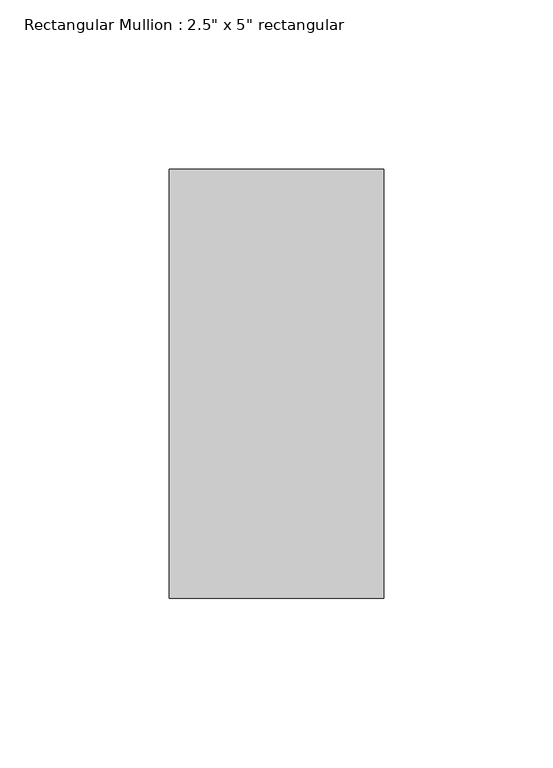
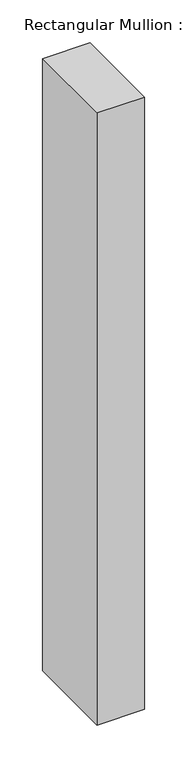
"""IFC4 building model written with IfcOpenShell, lengths in millimetres: member geometry."""

from ifc_helpers import new_model, si_unit, frame, origin, place, context, project, spatial, polyline, outline, extrude, source, transform, mapped, element, save


def member_5e57c25a(model_context):
    return source(origin(), model_context, "Body", "SweptSolid", [
        extrude(outline(polyline([(31.75, 63.5), (31.75, -63.5), (-31.75, -63.5), (-31.75, 63.5), (31.75, 63.5)])), frame((0.0, 0.0, -871.2851947), z_axis=(0.0, 0.0, 1.0), x_axis=(1.0, 0.0, 0.0)), (0.0, 0.0, 1.0), 871.2851947),
    ])


if __name__ == "__main__":
    model = new_model("IFC4")
    model_context = context("Model", 3, world=origin())
    ifc_project = project(units=[si_unit("LENGTHUNIT", "METRE", prefix="MILLI")], contexts=[model_context])
    site = spatial("IfcSite", under=ifc_project)
    building = spatial("IfcBuilding", under=site)
    placement = place(None, origin())
    member_shape = member_5e57c25a(model_context)
    element("IfcMember", 1, ObjectType="Rectangular Mullion : 2.5\" x 5\" rectangular", at=placement, inside=building, context=model_context, shape_type="MappedRepresentation", body=[
        mapped(member_shape, transform((0.0, 0.0, 0.0), x_axis=(1.0, 0.0, 0.0), y_axis=(0.0, 1.0, 0.0), z_axis=(0.0, 0.0, 1.0))),
    ])
    save(model, "model.ifc")

# Revit data of these elements
# Type "Rectangular Mullion : 2.5\" x 5\" rectangular"
#   built-in parameter 1007304 = 0.416667 (stored number, unit not read)
#   built-in parameter 1007301 = 0.104167 (stored number, unit not read)
#   built-in parameter 1007300 = 0.104167 (stored number, unit not read)
# Element 1 (IfcMember, "Rectangular Mullion : 2.5\" x 5\" rectangular")
#   Materials on its faces: "Aluminum"
# Materials
#   "Aluminum": class "Metal", colour RGB 247 247 247, transparency 0, Description = "Aluminum 6061", Cost = 0
